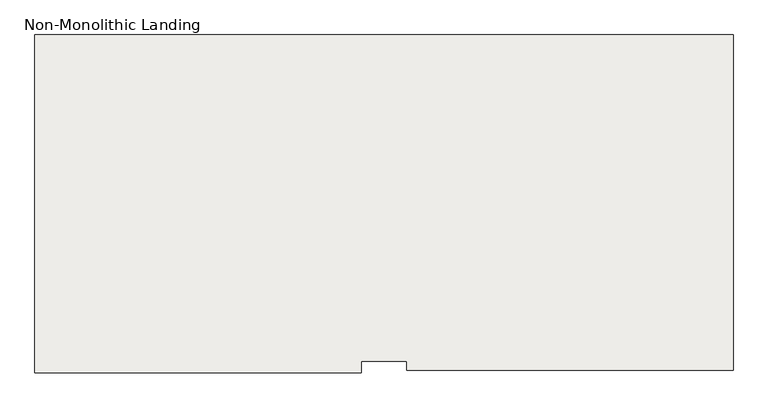
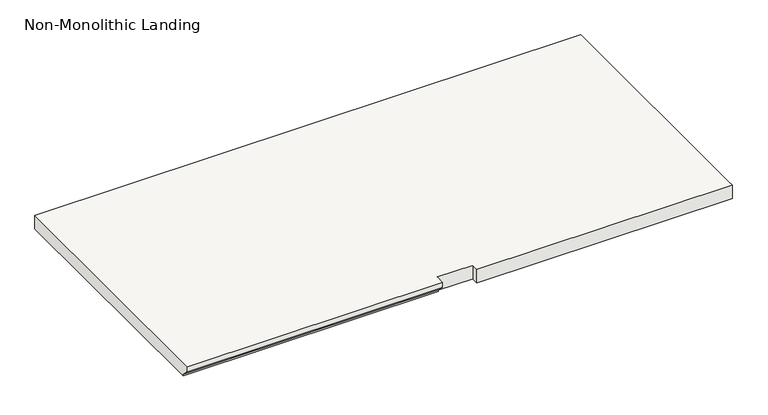
"""IFC4 building model written with IfcOpenShell, lengths in millimetres: slab geometry, Non-Monolithic Landing."""

from ifc_helpers import new_model, si_unit, origin, place, context, project, spatial, faceted_brep, source, transform, mapped, element, save


def non_monolithic_landing_0f5a95a9(model_context):
    return source(origin(), model_context, "Body", "Brep", [
        faceted_brep([(-9627.8771954, -2671.4727897, 4857.75), (-9627.8771954, -2671.4727897, 4876.8), (-10542.2771954, -2671.4727897, 4876.8), (-10542.2771954, -2671.4727897, 4857.75), (-9627.8771954, -2646.0727897, 4832.35), (-10542.2771954, -2646.0727897, 4832.35), (-9627.8771954, -2639.7227897, 4876.8), (-9500.8771954, -2639.7227897, 4876.8), (-9500.8771954, -2665.1227897, 4876.8), (-8586.4771954, -2665.1227897, 4876.8), (-8586.4771954, -2639.7227897, 4876.8), (-8586.4771954, -1725.3227897, 4876.8), (-10542.2771954, -1725.3227897, 4876.8), (-9627.8771954, -2646.0727897, 4826.0), (-10542.2771954, -2646.0727897, 4826.0), (-10542.2771954, -1725.3227897, 4826.0), (-8586.4771954, -1725.3227897, 4826.0), (-8586.4771954, -2639.7227897, 4826.0), (-8586.4771954, -2665.1227897, 4826.0), (-9500.8771954, -2665.1227897, 4826.0), (-9500.8771954, -2639.7227897, 4826.0), (-9627.8771954, -2639.7227897, 4826.0)], [[[0, 1, 2, 3]], [[4, 0, 3, 5]], [[6, 7, 8, 9, 10, 11, 12, 2, 1]], [[13, 14, 15, 16, 17, 18, 19, 20, 21]], [[14, 13, 4, 5]], [[6, 1, 0, 4, 13, 21]], [[7, 6, 21, 20]], [[8, 7, 20, 19]], [[9, 8, 19, 18]], [[10, 9, 18, 17]], [[11, 10, 17, 16]], [[12, 11, 16, 15]], [[2, 12, 15, 14, 5, 3]]]),
    ])


if __name__ == "__main__":
    model = new_model("IFC4")
    model_context = context("Model", 3, world=origin())
    ifc_project = project(units=[si_unit("LENGTHUNIT", "METRE", prefix="MILLI")], contexts=[model_context])
    site = spatial("IfcSite", under=ifc_project)
    building = spatial("IfcBuilding", under=site)
    placement = place(None, origin())
    non_monolithic_landing_shape = non_monolithic_landing_0f5a95a9(model_context)
    element("IfcSlab", 1, ObjectType="Non-Monolithic Landing", at=placement, inside=building, context=model_context, shape_type="MappedRepresentation", body=[
        mapped(non_monolithic_landing_shape, transform((0.0, 0.0, 0.0), x_axis=(1.0, 0.0, 0.0), y_axis=(0.0, 1.0, 0.0), z_axis=(0.0, 0.0, 1.0))),
    ])
    save(model, "model.ifc")
